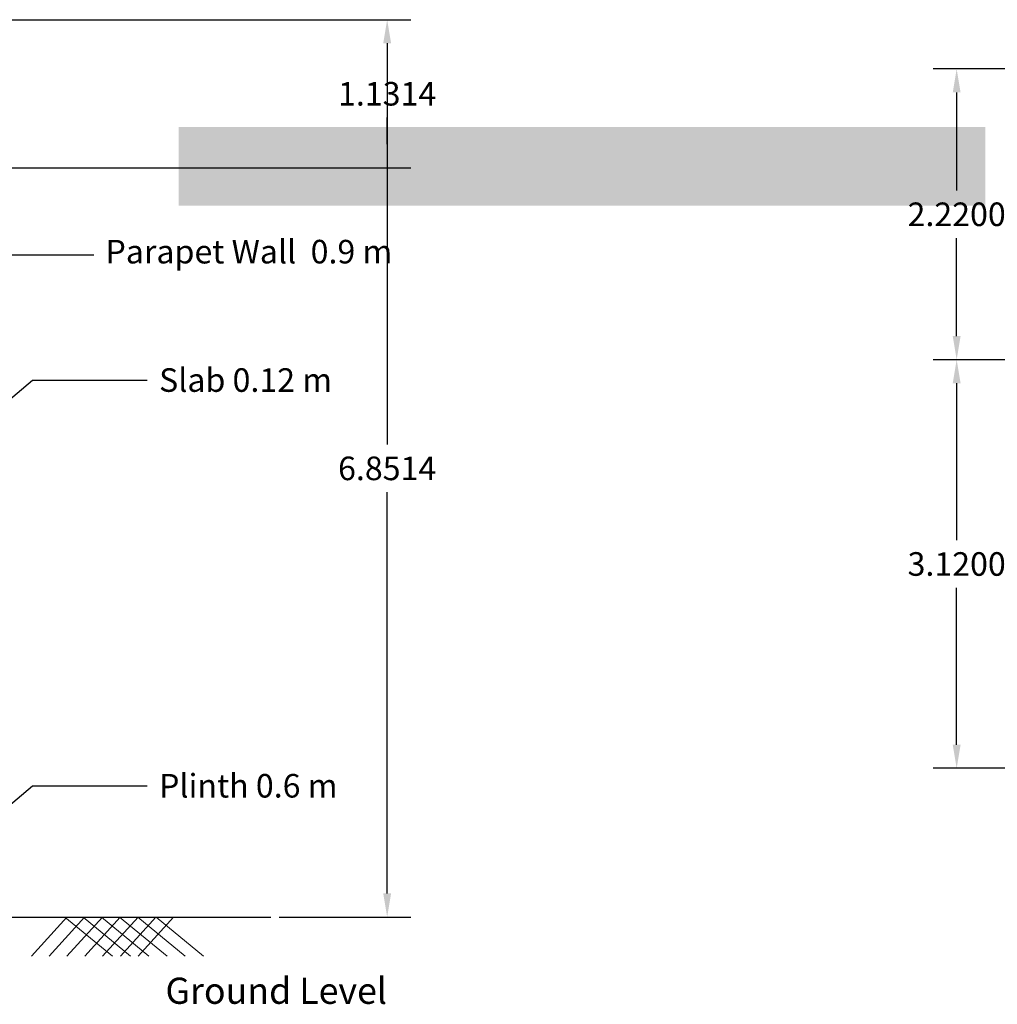
# Model space of a CAD drawing. Units: metres. Extents: x 5.2 to 41.7, y 12.2 to 37.4.
# Tile 5 of 6: x 19.4 to 26.9, y 28.8 to 36.3. Entities that reach past the tile are written whole.
import ezdxf
from ezdxf import colors
from ezdxf.entities.mleader import LeaderData, LeaderLine
from ezdxf.math import Vec2, Vec3

# ---------------------------------------------------------------- set-up
doc = ezdxf.new("R2010")
doc.units = ezdxf.units.M
doc.header["$MEASUREMENT"] = 0
for name, color, linetype, lineweight in [('A-ANNO-DIMS', 2, 'Continuous', 18), ('A-ANNO-TEXT', 3, 'Continuous', 18), ('C-TOPO', 7, 'Continuous', 25), ('C-TOPO-PATT', 8, 'Continuous', 13)]:
    doc.layers.add(name, color=color, linetype=linetype, lineweight=lineweight)
doc.layers.add('A-PLIN-PATT', color=251, linetype='Continuous', lineweight=13, true_color=0x636466)
doc.styles.get("Standard").update_dxf_attribs({"font": 'arial.ttf'})
doc.dimstyles.get("Standard").update_dxf_attribs({"dimtxt": 0.18, "dimasz": 0.18, "dimexe": 0.18, "dimexo": 0.0625, "dimgap": 0.09, "dimtad": 0, "dimtih": 1, "dimtoh": 1, "dimdec": 4, "dimzin": 0, "dimdsep": 46, "dimtxsty": 'Standard', "dimcen": 0.09, "dimadec": 0, "dimazin": 0, "dimtfac": 1, "dimtdec": 4, "dimtofl": 0, "dimtmove": 0, "dimatfit": 3, "dimfxl": 1, "dimtolj": 1, "dimtzin": 0, "dimarcsym": 0})

# ---------------------------------------------------------------- blocks, each defined once
blk = doc.blocks.new('*D38')
at = {"layer": 'A-ANNO-DIMS', "color": 0, "lineweight": -2, "transparency": 16777216}
for p, q in [((14.9621, 36.2961), (22.4246, 36.2961)), ((22.2446, 36.1161), (22.2446, 33.0523)), ((22.2446, 29.6247), (22.2446, 32.6885)), ((21.4196, 29.4447), (22.4246, 29.4447))]:
    blk.add_line(p, q, dxfattribs=at)
at = {"layer": 'A-ANNO-DIMS', "color": 0, "lineweight": 25, "transparency": 16777216}
for points in [[(22.2146, 36.1161), (22.2746, 36.1161), (22.2446, 36.2961)], [(22.2146, 29.6247), (22.2746, 29.6247), (22.2446, 29.4447)]]:
    blk.add_solid(points, dxfattribs=at)
at = {"layer": 'Defpoints', "color": 0, "lineweight": 25, "transparency": 16777216}
for p in [(14.8996, 36.2961), (22.2446, 36.2961), (21.3571, 29.4447)]:
    blk.add_point(p, dxfattribs=at)
at = {"layer": 'A-ANNO-DIMS', "color": 0, "transparency": 16777216, "insert": (22.2446, 32.8704), "char_height": 0.18, "attachment_point": 5}
blk.add_mtext('\\A1;6.8514', dxfattribs=at)
blk = doc.blocks.new('*D45')
at = {"layer": 'A-ANNO-DIMS', "color": 0, "lineweight": -2, "transparency": 16777216}
for p, q in [((14.9621, 36.2961), (22.4246, 36.2961)), ((22.2446, 36.1161), (22.2446, 35.9124)), ((22.2446, 35.3447), (22.2446, 35.5484)), ((14.6321, 35.1647), (22.4246, 35.1647))]:
    blk.add_line(p, q, dxfattribs=at)
at = {"layer": 'A-ANNO-DIMS', "color": 0, "lineweight": 25, "transparency": 16777216}
for points in [[(22.2146, 36.1161), (22.2746, 36.1161), (22.2446, 36.2961)], [(22.2146, 35.3447), (22.2746, 35.3447), (22.2446, 35.1647)]]:
    blk.add_solid(points, dxfattribs=at)
at = {"layer": 'Defpoints', "color": 0, "lineweight": 25, "transparency": 16777216}
for p in [(14.8996, 36.2961), (22.2446, 36.2961), (14.5696, 35.1647)]:
    blk.add_point(p, dxfattribs=at)
at = {"layer": 'A-ANNO-DIMS', "color": 0, "transparency": 16777216, "insert": (22.2446, 35.7304), "char_height": 0.18, "attachment_point": 5}
blk.add_mtext('\\A1;1.1314', dxfattribs=at)
blk = doc.blocks.new('*D50')
at = {"layer": 'A-ANNO-DIMS', "color": 0, "lineweight": -2, "transparency": 16777216}
for p, q in [((28.065, 33.7003), (26.413, 33.7003)), ((26.593, 33.5203), (26.593, 32.3222)), ((26.593, 30.7603), (26.593, 31.9583)), ((28.065, 30.5803), (26.413, 30.5803))]:
    blk.add_line(p, q, dxfattribs=at)
at = {"layer": 'A-ANNO-DIMS', "color": 0, "lineweight": 25, "transparency": 16777216}
for points in [[(26.563, 33.5203), (26.623, 33.5203), (26.593, 33.7003)], [(26.563, 30.7603), (26.623, 30.7603), (26.593, 30.5803)]]:
    blk.add_solid(points, dxfattribs=at)
at = {"layer": 'Defpoints', "color": 0, "lineweight": 25, "transparency": 16777216}
for p in [(26.593, 33.7003), (28.1275, 33.7003), (28.1275, 30.5803)]:
    blk.add_point(p, dxfattribs=at)
at = {"layer": 'A-ANNO-DIMS', "color": 0, "transparency": 16777216, "insert": (26.593, 32.1403), "char_height": 0.18, "attachment_point": 5}
blk.add_mtext('\\A1;3.1200', dxfattribs=at)
blk = doc.blocks.new('*D56')
at = {"layer": 'A-ANNO-DIMS', "color": 0, "lineweight": -2, "transparency": 16777216}
for p, q in [((31.885, 35.9203), (26.413, 35.9203)), ((26.593, 35.7403), (26.593, 34.9922)), ((26.593, 33.8803), (26.593, 34.6284)), ((31.985, 33.7003), (26.413, 33.7003))]:
    blk.add_line(p, q, dxfattribs=at)
at = {"layer": 'A-ANNO-DIMS', "color": 0, "lineweight": 25, "transparency": 16777216}
for points in [[(26.563, 35.7403), (26.623, 35.7403), (26.593, 35.9203)], [(26.563, 33.8803), (26.623, 33.8803), (26.593, 33.7003)]]:
    blk.add_solid(points, dxfattribs=at)
at = {"layer": 'Defpoints', "color": 0, "lineweight": 25, "transparency": 16777216}
for p in [(26.593, 35.9203), (31.9475, 35.9203), (32.0475, 33.7003)]:
    blk.add_point(p, dxfattribs=at)
at = {"layer": 'A-ANNO-DIMS', "color": 0, "transparency": 16777216, "insert": (26.593, 34.8103), "char_height": 0.18, "attachment_point": 5}
blk.add_mtext('\\A1;2.2200', dxfattribs=at)

msp = doc.modelspace()

# ---------------------------------------------------------------- hatches: boundary and pattern name
at = {"layer": 'A-PLIN-PATT'}
h = msp.add_hatch(dxfattribs=at)
h.set_pattern_fill('GRAVEL', color=256, scale=0.02)
h.set_pattern_definition([(228.0127875, (0.0144, 0.02), (-0.16, -0.18), [0.00269072, -0.266381761]), (184.9697407, (0.0126, 0.018), (0.24, 0.02), [0.00461736, -0.457118495]), (132.510447, (0.008, 0.0176), (0.2, -0.22), [0.00325576, -0.322320652]), (267.273689, (0.0002, 0.0126), (0.02, 0.4), [0.00420476, -0.416271161]), (292.8336542, (0, 0.0084), (-0.1, 0.24), [0.0041231, -0.4081874626]), (357.273689, (0.0016, 0.0046), (-0.4, 0.02), [0.00420476, -0.416271161]), (37.6942405, (0.0058, 0.0044), (-0.26, -0.2), [0.00556058, -0.550496971]), (72.2553284, (0.0102, 0.0078), (0.14, 0.44), [0.00524976, -0.51972643]), (121.4295656, (0.0118, 0.0128), (-0.16, 0.26), [0.004219, -0.417681462]), (175.2363583, (0.0096, 0.0164), (0.22, -0.02), [0.00481664, -0.2360152516]), (222.3974378, (0.0048, 0.0168), (-0.24, -0.22), [0.00622896, -0.6166675]), (138.814075, (0.02, 0.0124), (-0.14, 0.12), [0.00212602, -0.210476896]), (171.4692344, (0.0184, 0.0138), (0.26, -0.04), [0.00404474, -0.400430228]), (225, (0.0144, 0.0144), (0, -0.02), [0.00282842, -0.025455851]), (203.1985905, (0.013, 0.0168), (0.1, 0.04), [0.00152316, -0.150792302]), (291.8014095, (0.0116, 0.0162), (-0.02, 0.06), [0.00215406, -0.105549236]), (30.9637565, (0.0124, 0.0142), (0.06, 0.04), [0.00349858, -0.113120458]), (161.565051, (0.0154, 0.016), (0.04, -0.02), [0.00252982, -0.060715733]), (16.3895403, (0, 0.0162), (0.2, 0.06), [0.003544, -0.350856903]), (70.346176, (0.0034, 0.0172), (-0.08, -0.22), [0.00297322, -0.294348155]), (293.1985905, (0.0154, 0.02), (-0.04, 0.1), [0.0030463, -0.149269162]), (343.6104597, (0.0166, 0.0172), (-0.2, 0.06), [0.003544, -0.350856903]), (339.443955, (0, 0.0038), (-0.1, 0.04), [0.0034176, -0.167462475]), (294.7751406, (0.0032, 0.0026), (-0.1, 0.22), [0.00286356, -0.283492861]), (66.8014095, (0.0156, 0), (0.04, 0.1), [0.0030463, -0.149269162]), (17.3540246, (0.0168, 0.0028), (-0.26, -0.08), [0.00335262, -0.331908472]), (69.443955, (0.0058, 0), (-0.04, -0.1), [0.0017088, -0.169171275]), (101.309932, (0.0144, 0), (-0.02, 0.08), [0.0010198, -0.10096059]), (165.963757, (0.0142, 0.001), (0.06, -0.02), [0.0041231, -0.0783390125]), (186.009006, (0.0102, 0.002), (0.2, 0.02), [0.003821, -0.3782784635]), (303.690068, (0.0124, 0.0124), (-0.02, 0.04), [0.00288444, -0.0692265855]), (353.1572266, (0.014, 0.01), (0.34, -0.04), [0.00503588, -0.4985512525]), (60.945396, (0.019, 0.0094), (-0.08, -0.14), [0.00205912, -0.203853483]), (90, (0.02, 0.0112), (-0.02, 0.02), [0.0012, -0.0188]), (120.256437, (0.0098, 0.0026), (0.08, -0.14), [0.00277848, -0.2750704]), (48.0127875, (0.0084, 0.005), (0.16, 0.18), [0.00538144, -0.263691041]), (0, (0.012, 0.009), (0.02, 0.02), [0.0052, -0.0148]), (325.3048465, (0.0172, 0.009), (0.2, -0.14), [0.00316228, -0.313065486]), (254.054604, (0.0198, 0.0072), (-0.02, -0.08), [0.00291204, -0.142690158]), (207.6459754, (0.019, 0.0044), (-0.38, -0.2), [0.0047413, -0.469389484]), (175.4260787, (0.0148, 0.0022), (-0.26, 0.02), [0.00501598, -0.496581468])])
h.paths.add_polyline_path([(23.80317, 35.47718), (20.65317, 35.47718), (20.65317, 34.87718), (23.80317, 34.87718)])
h.paths.add_polyline_path([(26.81317, 35.47718), (26.71317, 35.47718), (23.80317, 35.47718), (23.80317, 34.87718), (26.81317, 34.87718)])
h.paths.add_polyline_path([(30.46113, 35.47718), (27.91317, 35.47718), (27.91317, 35.32718), (28.21317, 35.32718), (28.21317, 35.17718), (28.51317, 35.17718), (28.51317, 35.02718), (28.81317, 35.02718), (28.81317, 34.87718), (30.46113, 34.87718)])
h.paths.add_polyline_path([(30.96317, 35.47718), (30.76113, 35.47718), (30.76113, 34.87718), (30.96317, 34.87718)])
at = {"layer": 'C-TOPO-PATT'}
h = msp.add_hatch(dxfattribs=at)
h.set_pattern_fill('ANSI31', color=256, scale=0.80661, angle=2.9144, style=0)
h.paths.add_polyline_path([(19.49943, 29.1447), (20.34782, 29.1447), (20.61877, 29.44472), (19.77038, 29.44472)])
h = msp.add_hatch(dxfattribs=at)
h.set_pattern_fill('ANSI31', color=256, scale=0.709474, angle=95.361, style=0)
h.paths.add_polyline_path([(19.77038, 29.44472), (20.13254, 29.1447), (20.98093, 29.1447), (20.61877, 29.44472)])

# ---------------------------------------------------------------- linework, layer by layer
at = {"layer": 'C-TOPO'}
msp.add_line((19.04956, 29.44472), (21.3571, 29.44472), dxfattribs=at)

# ---------------------------------------------------------------- texts
at = {"layer": 'A-ANNO-TEXT', "insert": (20.47337, 28.98194), "char_height": 0.2, "attachment_point": 1}
msp.add_mtext_dynamic_manual_height_columns('\\pxqc;{Ground Level }', width=1.8483261, gutter_width=1, heights=[0], dxfattribs=at)

# ---------------------------------------------------------------- dimensions: what is measured, and where the dimension line sits
at = {"layer": 'A-ANNO-DIMS'}
for base, p1, p2, picture, middle in [((22.2446, 36.29608), (14.56956, 35.16472), (14.89956, 36.29608), '*D45', (22.2446, 35.7304)), ((22.2446, 36.29608), (21.3571, 29.44472), (14.89956, 36.29608), '*D38', (22.2446, 32.8704)), ((26.59298, 35.92026), (32.04748, 33.70026), (31.94748, 35.92026), '*D56', (26.59298, 34.81026)), ((26.59298, 33.70026), (28.12748, 30.58026), (28.12748, 33.70026), '*D50', (26.59298, 32.14026))]:
    dim = msp.add_linear_dim(base=base, p1=p1, p2=p2, angle=90, dimstyle='Standard', override={"dimdec": 4, "dimlfac": 1, "dimrnd": 0, "dimzin": 0, "dimdsep": 46, "dimlunit": 2}, dxfattribs=at)
    dim.commit()
    dim.dimension.update_dxf_attribs({"geometry": picture, "text_midpoint": middle})

# ---------------------------------------------------------------- leaders
at = {"layer": 'A-ANNO-TEXT'}
ml = msp.add_multileader_mtext('Standard', dxfattribs=at)
ml.set_content('Parapet Wall  0.9 m  ', color=256)
ml.set_leader_properties()
ml.build(insert=Vec2(0, 0))
ml.multileader.update_dxf_attribs({"dogleg_length": 0.36, "arrow_head_size": 0.18})
ctx = ml.context
ctx.base_point, ctx.char_height, ctx.arrow_head_size, ctx.landing_gap_size, ctx.plane_origin = Vec3(20.00372, 34.49999), 0.18, 0.18, 0.09, Vec3(18.71195, 33.97238)
notes = []
notes.append((ctx, [(0, (1, 1, 0), (19.12675, 34.49999), (1, 0), 0.87697, [(0, [(18.78338, 34.07758)], 0, [])])]))
ctx.mtext.insert, ctx.mtext.flow_direction = Vec3(20.09372, 34.61498), 5
ml = msp.add_multileader_mtext('Standard', dxfattribs=at)
ml.set_content('Slab 0.12 m   ', color=256)
ml.set_leader_properties()
ml.build(insert=Vec2(0, 0))
ml.multileader.update_dxf_attribs({"dogleg_length": 0.36, "arrow_head_size": 0.18})
ctx = ml.context
ctx.base_point, ctx.char_height, ctx.arrow_head_size, ctx.landing_gap_size, ctx.plane_origin = Vec3(20.41302, 33.54318), 0.18, 0.18, 0.09, Vec3(18.94271, 32.33032)
notes.append((ctx, [(0, (1, 1, 0), (19.53605, 33.54318), (1, 0), 0.87697, [(0, [(19.09956, 33.17607)], 0, [])])]))
ctx.mtext.insert, ctx.mtext.flow_direction = Vec3(20.50302, 33.63471), 5
ml = msp.add_multileader_mtext('Standard', dxfattribs=at)
ml.set_content('Plinth 0.6 m   ', color=256)
ml.set_leader_properties()
ml.build(insert=Vec2(0, 0))
ml.multileader.update_dxf_attribs({"dogleg_length": 0.36, "arrow_head_size": 0.18})
ctx = ml.context
ctx.base_point, ctx.char_height, ctx.arrow_head_size, ctx.landing_gap_size, ctx.plane_origin = Vec3(20.41302, 30.44541), 0.18, 0.18, 0.09, Vec3(18.94271, 29.23256)
notes.append((ctx, [(0, (1, 1, 0), (19.53605, 30.44541), (1, 0), 0.87697, [(0, [(19.09956, 30.07831)], 0, [])])]))
ctx.mtext.insert, ctx.mtext.flow_direction = Vec3(20.50302, 30.53695), 5
for ctx, leaders in notes:
    for number, flags, end, landing, length, lines in leaders:
        leader = LeaderData()
        leader.index, (leader.has_last_leader_line, leader.has_dogleg_vector, leader.attachment_direction) = number, flags
        leader.last_leader_point, leader.dogleg_vector, leader.dogleg_length = Vec3(end), Vec3(landing), length
        for number, points, colour, breaks in lines:
            line = LeaderLine()
            line.index, line.vertices, line.color, line.breaks = number, Vec3.list(points), colors.encode_raw_color(colour), breaks
            leader.lines.append(line)
        ctx.leaders.append(leader)

doc.saveas('drawing.dxf')
